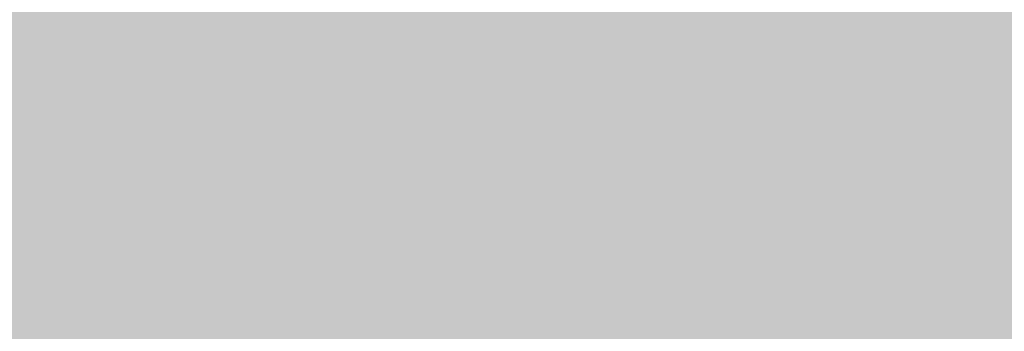
# Model space of a CAD drawing. Units: inches. Extents: x 2083 to 3317, y 1141 to 2115.
# Tile 142 of 256: x 3126.6699 to 3126.8176, y 1263.3081 to 1263.3548. Entities that reach past the tile are written whole.
import ezdxf

# ---------------------------------------------------------------- set-up
doc = ezdxf.new("R2010")
doc.units = ezdxf.units.IN
doc.layers.add('A-ANNO-DIMS', color=2, linetype='Continuous', lineweight=18)
doc.layers.add('A-WALL-PATT', color=251, linetype='Continuous', lineweight=13, true_color=0x636466)
doc.styles.get("Standard").update_dxf_attribs({"font": 'arial.ttf'})
doc.dimstyles.new('ISO-25', dxfattribs={"dimtxt": 12, "dimasz": 12, "dimexe": 1.25, "dimexo": 0.625, "dimtad": 1, "dimlunit": 3, "dimtxsty": 'Standard', "dimcen": 2.5, "dimadec": 0, "dimazin": 0, "dimtfac": 1, "dimtmove": 0, "dimatfit": 3, "dimfxl": 1, "dimarcsym": 0})

# ---------------------------------------------------------------- blocks, each defined once
blk = doc.blocks.new('*D26')
at = {"layer": 'A-ANNO-DIMS', "color": 0, "lineweight": -2, "transparency": 16777216}
for p, q in [((3088.98584, 1274.91509), (3088.98584, 1270.95196)), ((3111.24004, 1274.91509), (3111.24004, 1270.95196)), ((3076.98584, 1272.20196), (2840.26245, 1272.20196)), ((3111.24004, 1272.20196), (3088.98584, 1272.20196)), ((3123.24004, 1272.20196), (3135.24004, 1272.20196))]:
    blk.add_line(p, q, dxfattribs=at)
at = {"layer": 'A-ANNO-DIMS', "color": 0, "transparency": 16777216}
for points in [[(3076.98584, 1274.20196), (3076.98584, 1270.20196), (3088.98584, 1272.20196)], [(3123.24004, 1274.20196), (3123.24004, 1270.20196), (3111.24004, 1272.20196)]]:
    blk.add_solid(points, dxfattribs=at)
at = {"layer": 'Defpoints', "color": 0, "transparency": 16777216}
for p in [(3088.98584, 1275.54009), (3111.24004, 1275.54009), (3088.98584, 1272.20196)]:
    blk.add_point(p, dxfattribs=at)
at = {"layer": 'A-ANNO-DIMS', "color": 0, "transparency": 16777216, "insert": (2952.62415, 1279.0316), "char_height": 12, "attachment_point": 5}
blk.add_mtext('NIGHTSTAND 1\'-10 1/2" TYP.', dxfattribs=at)
blk = doc.blocks.new('*D27')
at = {"layer": 'A-ANNO-DIMS', "color": 0, "lineweight": -2, "transparency": 16777216}
for p, q in [((3114.57817, 1309.79428), (3114.57817, 1321.79428)), ((3111.86504, 1297.79428), (3115.82817, 1297.79428)), ((3114.57817, 1297.79428), (3114.57817, 1275.54009)), ((3111.86504, 1275.54009), (3115.82817, 1275.54009)), ((3114.57817, 1263.54009), (3114.57817, 1140.98859))]:
    blk.add_line(p, q, dxfattribs=at)
at = {"layer": 'A-ANNO-DIMS', "color": 0, "transparency": 16777216}
for points in [[(3112.57817, 1309.79428), (3116.57817, 1309.79428), (3114.57817, 1297.79428)], [(3112.57817, 1263.54009), (3116.57817, 1263.54009), (3114.57817, 1275.54009)]]:
    blk.add_solid(points, dxfattribs=at)
at = {"layer": 'Defpoints', "color": 0, "transparency": 16777216}
for p in [(3111.24004, 1297.79428), (3111.24004, 1275.54009), (3114.57817, 1275.54009)]:
    blk.add_point(p, dxfattribs=at)
at = {"layer": 'A-ANNO-DIMS', "color": 0, "transparency": 16777216, "insert": (3107.74853, 1196.26434), "char_height": 12, "attachment_point": 5, "rotation": 90}
blk.add_mtext('1\'-10 1/2" TYP.', dxfattribs=at)

msp = doc.modelspace()

# ---------------------------------------------------------------- hatches: boundary and pattern name
at = {"layer": 'A-WALL-PATT'}
h = msp.add_hatch(color=256, dxfattribs=at)
h.dxf.hatch_style = 1
h.paths.add_polyline_path([(3126.95978, 2020.76136), (2748.95978, 2020.76136), (2604.95978, 2020.76136), (2226.95978, 2020.76136), (2226.95978, 1702.76136), (2466.95978, 1702.76136), (2466.95978, 1582.76136), (2418.95978, 1582.76136), (2418.95978, 1477.76136), (2226.95978, 1477.76136), (2226.95978, 1263.26136), (2544.95978, 1263.26136), (2544.95978, 1411.76136), (2604.95978, 1411.76136), (2685.95978, 1411.76136), (2685.95978, 1420.76136), (2604.95978, 1420.76136), (2604.95978, 1573.76136), (2604.95978, 1702.76136), (2604.95978, 2011.76136), (2748.95978, 2011.76136), (2748.95978, 1702.76136), (2862.95978, 1702.76136), (2862.95978, 1621.76136), (2871.95978, 1621.76136), (2871.95978, 1702.76136), (2883.95978, 1702.76136), (2883.95978, 1706.93946, -0.026459), (2883.95978, 1711.76136), (2757.95978, 1711.76136), (2757.95978, 1807.76136), (2787.95978, 1807.76136), (2787.95978, 1812.26136), (2757.95978, 1812.26136), (2757.95978, 2011.76136), (2877.95978, 2011.76136), (2877.95978, 1812.26136), (2847.95978, 1812.26136), (2847.95978, 1807.76136), (2889.83574, 1807.76136), (2889.83574, 1812.26136), (2882.45978, 1812.26136), (2882.45978, 2011.76136), (3117.95978, 2011.76136), (3117.95978, 1812.26136), (2937.83574, 1812.26136), (2937.83574, 1807.76136), (2995.70978, 1807.76136), (2995.70978, 1796.11767), (3000.20978, 1796.11767), (3000.20978, 1807.76136), (3117.95978, 1807.76136), (3117.95978, 1711.76136), (3000.20978, 1711.76136), (3000.20978, 1760.11767), (2998.5727, 1760.11767, -0.020711), (2995.70978, 1760.11767), (2995.70978, 1711.76136), (2931.95978, 1711.76136), (2931.95978, 1702.76136), (3126.95978, 1702.76136)])
h.paths.add_polyline_path([(2471.45978, 2011.76136), (2471.45978, 1810.01136), (2462.71694, 1810.01136), (2462.71694, 1805.51136), (2505.95978, 1805.51136), (2505.95978, 1810.01136), (2475.95978, 1810.01136), (2475.95978, 2011.76136), (2595.95978, 2011.76136), (2595.95978, 1810.01136), (2565.95978, 1810.01136), (2565.95978, 1805.51136), (2595.95978, 1805.51136), (2595.95978, 1711.76136), (2235.95978, 1711.76136), (2235.95978, 1805.51136), (2353.70978, 1805.51136), (2353.70978, 1796.05416), (2358.20978, 1796.05416), (2358.20978, 1805.51136), (2414.71694, 1805.51136), (2414.71694, 1810.01136), (2235.95978, 1810.01136), (2235.95978, 2011.76136)], flags=16)
h.paths.add_polyline_path([(2270.20473, 1994.61001), (2270.20473, 1970.61001), (2246.20473, 1970.61001), (2246.20473, 1994.61001)], flags=0)
edge = h.paths.add_edge_path(flags=0)
edge.add_ellipse((2332.02739, 1899.79818), major_axis=(-3.04299, 3.04299), ratio=0.1682525, start_angle=-161.33217, end_angle=-156.30711, ccw=False)
edge.add_ellipse((2333.08204, 1898.74353), major_axis=(-1.05465, 1.05465), ratio=0.4535321, start_angle=-123.37102, end_angle=-94.15911)
edge = h.paths.add_edge_path(flags=0)
edge.add_ellipse((2332.02739, 1968.87629), major_axis=(3.04299, 3.04299), ratio=0.1682525, start_angle=18.66783, end_angle=23.69289)
edge.add_spline(control_points=[(2332.9256, 1970.6911), (2332.22677, 1970.3361), (2330.89371, 1969.65891), (2328.41308, 1970.93214), (2327.20393, 1967.74871), (2324.7096, 1969.95559), (2322.53282, 1967.01235), (2320.01285, 1971.29581), (2317.68031, 1968.15784), (2316.04053, 1967.10205), (2315.4269, 1966.8096)], knot_values=[0, 0, 0, 0, 2.267059, 4.324559, 6.685584, 8.878641, 11.121502, 14.300359, 17.755284, 19.732645, 19.732645, 19.732645, 19.732645], degree=3, periodic=0)
edge.add_ellipse((2332.02739, 1968.87629), major_axis=(3.04299, 3.04299), ratio=0.1682525, start_angle=18.66783, end_angle=23.69289, ccw=False)
edge.add_ellipse((2333.08204, 1969.93094), major_axis=(1.05465, 1.05465), ratio=0.4535321, start_angle=56.62898, end_angle=85.84089, ccw=False)
edge = h.paths.add_edge_path(flags=0)
edge.add_spline(control_points=[(2296.42829, 1967.98791), (2293.6278, 1965.33631), (2287.70362, 1959.72709), (2299.74386, 1949.9957), (2294.53259, 1935.66853), (2290.57323, 1920.60351), (2293.39412, 1909.97369), (2296.18541, 1904.96654)], knot_values=[0.099185, 0.099185, 0.099185, 0.099185, 0.345301, 0.619822, 0.982653, 1.386093, 1.810555, 1.810555, 1.810555, 1.810555], degree=3, periodic=0)
edge.add_spline(control_points=[(2296.18541, 1904.96654), (2297.38358, 1902.6193), (2298.00097, 1901.94931), (2298.55297, 1901.46815)], knot_values=[0.006246, 0.006246, 0.006246, 0.006246, 0.055476, 0.055476, 0.055476, 0.055476], degree=3, periodic=0)
edge.add_spline(control_points=[(2298.55297, 1901.46815), (2297.25861, 1900.92322), (2295.22529, 1900.23213), (2293.06023, 1900.61421), (2292.10142, 1900.78841), (2292.08958, 1900.79057)], knot_values=[0.312835, 0.312835, 0.312835, 0.312835, 0.40178, 0.474987, 0.475903, 0.475903, 0.475903, 0.475903], degree=3, periodic=0)
edge.add_arc((2292.79365, 1904.66411), 3.93701, 215.4209, 259.69818, ccw=False)
edge.add_spline(control_points=[(2289.58531, 1902.3823), (2289.47665, 1902.53509), (2289.36848, 1902.68804), (2289.26086, 1902.84117)], knot_values=[0.102872, 0.102872, 0.102872, 0.102872, 0.116896, 0.116896, 0.116896, 0.116896], degree=3, periodic=0)
edge.add_spline(control_points=[(2289.26086, 1902.84117), (2288.6866, 1902.55019), (2287.64005, 1902.0199), (2285.88134, 1901.87395), (2283.85297, 1901.50435), (2281.71999, 1899.71054), (2278.46699, 1899.49294), (2276.15714, 1901.8832), (2272.25895, 1899.80407), (2267.77761, 1901.84318), (2262.24388, 1900.18403), (2257.41493, 1901.78206), (2254.31837, 1900.72612), (2253.17828, 1900.33734)], knot_values=[0, 0, 0, 0, 1.907977, 3.477176, 5.261074, 7.972851, 11.680248, 13.717921, 16.939592, 22.789562, 27.502503, 33.595215, 37.145618, 37.145618, 37.145618, 37.145618], degree=3, periodic=0)
edge.add_line((2253.17828, 1900.33734), (2250.24424, 1902.84117))
edge.add_line((2250.24424, 1902.84117), (2250.24424, 1965.8333))
edge.add_line((2250.24424, 1965.8333), (2253.17828, 1968.33712))
edge.add_spline(control_points=[(2253.17828, 1968.33712), (2254.31837, 1967.94835), (2257.41493, 1966.89241), (2262.24388, 1968.49043), (2267.77761, 1966.83128), (2271.52673, 1968.53722), (2273.87591, 1967.82829), (2274.2067, 1967.72764)], knot_values=[0, 0, 0, 0, 0.09018, 0.244935, 0.364644, 0.513233, 0.537855, 0.537855, 0.537855, 0.537855], degree=3, periodic=0)
edge.add_arc((2274.35289, 1963.79335), 3.93701, 72.05113, 92.12795, ccw=False)
edge.add_arc((2281.29693, 1985.23), 18.5963, 252.051134, 288.565722)
edge.add_arc((2292.31672, 1956.02888), 12.64608, 71.026788, 113.778218, ccw=False)
edge = h.paths.add_edge_path(flags=0)
edge.add_spline(control_points=[(2274.89941, 1951.85619), (2275.06616, 1951.61659), (2275.23269, 1951.37659), (2275.39799, 1951.13585)], knot_values=[1.409916, 1.409916, 1.409916, 1.409916, 1.43159, 1.43159, 1.43159, 1.43159], degree=3, periodic=0)
edge.add_spline(control_points=[(2275.39799, 1951.13585), (2275.79211, 1950.56189), (2276.17923, 1949.98377), (2276.54555, 1949.3971)], knot_values=[1.358238, 1.358238, 1.358238, 1.358238, 1.409916, 1.409916, 1.409916, 1.409916], degree=3, periodic=0)
edge.add_line((2276.54555, 1949.3971), (2277.43729, 1947.86218))
edge.add_spline(control_points=[(2277.43729, 1947.86218), (2276.30383, 1945.67311), (2274.6397, 1942.42688), (2274.63161, 1938.0939), (2272.79912, 1930.85155), (2274.35643, 1943.89705), (2275.94768, 1947.92336), (2276.54555, 1949.3971)], knot_values=[0.005632, 0.005632, 0.005632, 0.005632, 0.186014, 0.266002, 0.357087, 0.59639, 0.739732, 0.739732, 0.739732, 0.739732], degree=3, periodic=0)
edge.add_spline(control_points=[(2276.54555, 1949.3971), (2276.17923, 1949.98377), (2275.79211, 1950.56189), (2275.39799, 1951.13585)], knot_values=[1.358238, 1.358238, 1.358238, 1.358238, 1.409916, 1.409916, 1.409916, 1.409916], degree=3, periodic=0)
edge.add_spline(control_points=[(2275.39799, 1951.13585), (2274.9425, 1950.08045), (2274.20776, 1948.02527), (2273.9346, 1944.85148), (2272.46853, 1937.62749), (2273.46622, 1945.69647), (2274.70062, 1951.05947), (2274.89941, 1951.85619)], knot_values=[0.104364, 0.104364, 0.104364, 0.104364, 0.189636, 0.269624, 0.36071, 0.600013, 0.644622, 0.644622, 0.644622, 0.644622], degree=3, periodic=0)
h.paths.add_polyline_path([(2269.16751, 1963.12757, -0.357527), (2268.17063, 1960.97637, -0.092561), (2268.17063, 1939.43632, -0.357527), (2269.16751, 1937.28512, -0.357527), (2267.01631, 1938.282, -0.164785), (2254.68558, 1938.282, -0.357527), (2252.53438, 1937.28512, -0.357527), (2253.53126, 1939.43632, -0.092561), (2253.53126, 1960.97637, -0.357527), (2252.53438, 1963.12757, -0.357527), (2254.68558, 1962.13069, -0.164785), (2267.01631, 1962.13069, -0.357527)], flags=0)
h.paths.add_polyline_path([(2248.87407, 1967.8018), (2248.87407, 1957.02771), (2249.45778, 1957.02771), (2249.45778, 1911.64676), (2248.87407, 1911.64676), (2248.87407, 1900.87267), (2246.51186, 1900.87267, 0.197327), (2244.14966, 1902.45687), (2244.14966, 1966.21759, 0.197327), (2246.51186, 1967.8018)], flags=0)
h.paths.add_polyline_path([(2269.16751, 1931.38934, -0.357527), (2268.17063, 1929.23814, -0.092561), (2268.17063, 1907.6981, -0.357527), (2269.16751, 1905.54689, -0.357527), (2267.01631, 1906.54377, -0.164785), (2254.68558, 1906.54377, -0.357527), (2252.53438, 1905.54689, -0.357527), (2253.53126, 1907.6981, -0.092561), (2253.53126, 1929.23814, -0.357527), (2252.53438, 1931.38934, -0.357527), (2254.68558, 1930.39246, -0.164785), (2267.01631, 1930.39246, -0.357527)], flags=0)
edge = h.paths.add_edge_path(flags=0)
edge.add_spline(control_points=[(2276.19686, 1906.7237), (2276.16814, 1909.02893), (2276.11405, 1913.37185), (2270.59842, 1924.92498), (2273.90517, 1919.01278), (2275.92171, 1916.26206), (2275.47457, 1912.40215), (2277.25787, 1910.38062), (2276.69604, 1908.22504), (2276.64622, 1906.81302), (2276.61782, 1906.00841)], knot_values=[0, 0, 0, 0, 8.61026, 16.221274, 18.843057, 23.804898, 27.440828, 29.356102, 31.203478, 33.650687, 33.650687, 33.650687, 33.650687], degree=3, periodic=0)
edge.add_spline(control_points=[(2276.61782, 1906.00841), (2276.62331, 1905.62414), (2276.49774, 1904.62866), (2275.44178, 1903.85473), (2274.93731, 1903.08045), (2274.85908, 1902.84117)], knot_values=[0.156488, 0.156488, 0.156488, 0.156488, 0.184398, 0.231376, 0.250598, 0.250598, 0.250598, 0.250598], degree=3, periodic=0)
edge.add_line((2274.85908, 1902.84117), (2276.50598, 1902.84117))
edge.add_spline(control_points=[(2276.50598, 1902.84117), (2276.78831, 1903.08494), (2277.66507, 1904.1252), (2278.24954, 1904.34074), (2277.65387, 1908.52739), (2278.15567, 1906.22781), (2278.10046, 1905.28595), (2278.84667, 1904.06901), (2277.85679, 1903.41495), (2277.87419, 1902.99105), (2277.90356, 1902.84117)], knot_values=[0.059574, 0.059574, 0.059574, 0.059574, 0.080753, 0.103741, 0.16972, 0.176036, 0.207137, 0.240474, 0.262341, 0.27366, 0.27366, 0.27366, 0.27366], degree=3, periodic=0)
edge.add_line((2277.90356, 1902.84117), (2280.02983, 1902.84117))
edge.add_spline(control_points=[(2280.02983, 1902.84117), (2279.88822, 1903.0884), (2279.49926, 1903.98155), (2280.15228, 1905.93935), (2278.10362, 1909.65776), (2279.76239, 1907.18529), (2280.3279, 1904.87486), (2280.48511, 1903.48959), (2281.46327, 1903.24943), (2281.75834, 1902.9365), (2281.83404, 1902.84117)], knot_values=[0.013856, 0.013856, 0.013856, 0.013856, 0.034874, 0.088867, 0.107879, 0.126738, 0.158714, 0.193757, 0.217487, 0.226722, 0.226722, 0.226722, 0.226722], degree=3, periodic=0)
edge.add_spline(control_points=[(2281.83404, 1902.84117), (2281.78753, 1902.8267), (2281.64702, 1902.78299), (2281.39553, 1902.85949), (2281.08808, 1902.98524), (2280.72068, 1903.0609), (2280.33345, 1903.02573), (2280.12477, 1902.89888), (2280.02983, 1902.84117)], knot_values=[0, 0, 0, 0, 0.14413, 0.435517, 0.749276, 1.153046, 1.548371, 1.878348, 1.878348, 1.878348, 1.878348], degree=3, periodic=0)
edge.add_line((2280.02983, 1902.84117), (2277.90356, 1902.84117))
edge.add_spline(control_points=[(2277.90356, 1902.84117), (2277.89286, 1902.79586), (2277.8654, 1902.67964), (2277.60748, 1902.68748), (2277.27405, 1902.8007), (2276.83792, 1902.61977), (2276.58381, 1902.78926), (2276.50598, 1902.84117)], knot_values=[0, 0, 0, 0, 0.127189, 0.326199, 0.628009, 1.24357, 1.515331, 1.515331, 1.515331, 1.515331], degree=3, periodic=0)
edge.add_line((2276.50598, 1902.84117), (2274.85908, 1902.84117))
edge.add_spline(control_points=[(2274.85908, 1902.84117), (2274.81444, 1902.89859), (2274.72513, 1903.01345), (2274.49348, 1903.11897), (2274.24429, 1902.96054), (2273.93712, 1903.18494), (2273.61404, 1902.98314), (2273.40832, 1902.88304), (2273.32225, 1902.84117)], knot_values=[0, 0, 0, 0, 0.21843, 0.436957, 0.687977, 0.990379, 1.398396, 1.69185, 1.69185, 1.69185, 1.69185], degree=3, periodic=0)
edge.add_spline(control_points=[(2273.32225, 1902.84117), (2273.61674, 1903.44569), (2274.274, 1904.53825), (2276.02724, 1904.5737), (2276.20696, 1906.58364), (2276.19686, 1906.7237)], knot_values=[0.012227, 0.012227, 0.012227, 0.012227, 0.059472, 0.106218, 0.134458, 0.134458, 0.134458, 0.134458], degree=3, periodic=0)
h.paths.add_polyline_path([(2270.77605, 1897.78983), (2270.77605, 1873.78983), (2246.77605, 1873.78983), (2246.77605, 1897.78983)], flags=0)
h.paths.add_polyline_path([(2353.70978, 1760.00506), (2353.70978, 1760.05416), (2358.20978, 1760.05416, -0.033729)], flags=0)
h.paths.add_polyline_path([(2321.81912, 1737.52919), (2341.99533, 1737.52919, -0.414214), (2343.20327, 1736.32124), (2343.20327, 1721.0206, -0.414214), (2341.99533, 1719.81265), (2321.81912, 1719.81265, -0.414214), (2320.61117, 1721.0206), (2320.61117, 1736.32124, -0.414214)], flags=0)
h.paths.add_polyline_path([(2324.23501, 1736.32124), (2339.57944, 1736.32124, -0.414214), (2341.99533, 1733.90535), (2341.99533, 1725.44973, -0.414214), (2339.57944, 1723.03384), (2333.68059, 1723.03384), (2333.84532, 1722.04547, -0.870646), (2335.4254, 1721.82589, -0.767327), (2333.92269, 1721.42324), (2331.29102, 1721.42324, -0.767327), (2329.78832, 1721.82589, -0.870646), (2331.3684, 1722.04547), (2331.53313, 1723.03384), (2324.23501, 1723.03384, -0.414214), (2321.81912, 1725.44973), (2321.81912, 1733.90535, -0.414214)], flags=0)
h.paths.add_polyline_path([(2570.48379, 1928.61544), (2589.68379, 1928.61544), (2590.16883, 1928.61544), (2590.16883, 1904.9934), (2570.48379, 1904.9934)], flags=0)
h.paths.add_polyline_path([(2574.44732, 1927.26382, -1), (2572.82884, 1927.26382, -1)], flags=0)
h.paths.add_polyline_path([(2573.08987, 1926.94088), (2573.92503, 1927.77604), (2574.14774, 1927.55333), (2573.31258, 1926.71817)], flags=0)
h.paths.add_polyline_path([(2578.77906, 1919.72962, -1), (2571.59166, 1919.72962, -1)], flags=0)
h.paths.add_polyline_path([(2578.38536, 1919.72962, -1), (2571.98536, 1919.72962, -1)], flags=0)
h.paths.add_polyline_path([(2331.59576, 1729.47622, -1), (2333.61795, 1729.47622, -1)], flags=0)
h.paths.add_polyline_path([(2578.03423, 1927.26382, -1), (2576.41574, 1927.26382, -1)], flags=0)
h.paths.add_polyline_path([(2576.68885, 1927.53109), (2576.91156, 1927.7538), (2577.74673, 1926.91863), (2577.52402, 1926.69592)], flags=0)
h.paths.add_polyline_path([(2578.13906, 1909.85954, -1), (2572.23166, 1909.85954, -1)], flags=0)
h.paths.add_polyline_path([(2577.74536, 1909.85954, -1), (2572.62536, 1909.85954, -1)], flags=0)
h.paths.add_polyline_path([(2583.79772, 1927.26382, -1), (2582.17923, 1927.26382, -1)], flags=0)
h.paths.add_polyline_path([(2582.71865, 1927.7538), (2583.55381, 1926.91863), (2583.3311, 1926.69592), (2582.49594, 1927.53109)], flags=0)
h.paths.add_polyline_path([(2582.49594, 1927.53109), (2582.71865, 1927.7538), (2583.55381, 1926.91863), (2583.3311, 1926.69592)], flags=0)
h.paths.add_polyline_path([(2587.73906, 1920.52962, -1), (2581.83166, 1920.52962, -1)], flags=0)
h.paths.add_polyline_path([(2587.34536, 1920.52962, -1), (2582.22536, 1920.52962, -1)], flags=0)
h.paths.add_polyline_path([(2587.38462, 1927.26382, -1), (2585.76613, 1927.26382, -1)], flags=0)
h.paths.add_polyline_path([(2586.08199, 1926.98025), (2586.91716, 1927.81541), (2587.13987, 1927.5927), (2586.3047, 1926.75754)], flags=0)
h.paths.add_polyline_path([(2588.37906, 1910.65954, -1), (2581.19166, 1910.65954, -1)], flags=0)
h.paths.add_polyline_path([(2587.98536, 1910.65954, -1), (2581.58536, 1910.65954, -1)], flags=0)
h.paths.add_polyline_path([(2417.16773, 1729.4779), (2437.34394, 1729.4779, -0.414214), (2438.55188, 1728.26995), (2438.55188, 1712.96931, -0.414214), (2437.34394, 1711.76136), (2417.16773, 1711.76136, -0.414214), (2415.95978, 1712.96931), (2415.95978, 1728.26995, -0.414214)], flags=0)
h.paths.add_polyline_path([(2419.58362, 1728.26995), (2434.92805, 1728.26995, -0.414214), (2437.34394, 1725.85406), (2437.34394, 1717.39844, -0.414214), (2434.92805, 1714.98255), (2429.0292, 1714.98255), (2429.19393, 1713.99418, -0.870646), (2430.77401, 1713.7746, -0.767327), (2429.2713, 1713.37195), (2426.63963, 1713.37195, -0.767327), (2425.13693, 1713.7746, -0.870646), (2426.71701, 1713.99418), (2426.88174, 1714.98255), (2419.58362, 1714.98255, -0.414214), (2417.16773, 1717.39844), (2417.16773, 1725.85406, -0.414214)], flags=0)
h.paths.add_polyline_path([(2419.58362, 1728.26995), (2434.92805, 1728.26995, -0.414214), (2437.34394, 1725.85406), (2437.34394, 1717.39844, -0.414214), (2434.92805, 1714.98255), (2429.0292, 1714.98255), (2428.35812, 1719.00903), (2427.55282, 1719.00903), (2426.88174, 1714.98255), (2419.58362, 1714.98255, -0.414214), (2417.16773, 1717.39844), (2417.16773, 1725.85406, -0.414214)], flags=0)
h.paths.add_polyline_path([(2426.94437, 1721.42492, -1), (2428.96656, 1721.42492, -1)], flags=0)
h.paths.add_polyline_path([(2475.95978, 1702.76136), (2595.95978, 1702.76136), (2595.95978, 1582.76136), (2475.95978, 1582.76136)], flags=16)
h.paths.add_polyline_path([(2427.95978, 1573.76136), (2595.95978, 1573.76136), (2595.95978, 1468.76136), (2595.95978, 1420.76136), (2384.45978, 1420.76136), (2384.45978, 1468.76136), (2427.95978, 1468.76136)], flags=16)
h.paths.add_polyline_path([(2379.95978, 1468.76136), (2379.95978, 1420.76136), (2235.95978, 1420.76136), (2235.95978, 1468.76136)], flags=16)
h.paths.add_polyline_path([(2317.816, 1466.69577), (2337.9922, 1466.69577, -0.414214), (2339.20015, 1465.48782), (2339.20015, 1450.18718, -0.414214), (2337.9922, 1448.97923), (2317.816, 1448.97923, -0.414214), (2316.60805, 1450.18718), (2316.60805, 1465.48782, -0.414214)], flags=0)
h.paths.add_polyline_path([(2320.23189, 1465.48782), (2335.57631, 1465.48782, -0.414214), (2337.9922, 1463.07193), (2337.9922, 1454.61631, -0.414214), (2335.57631, 1452.20042), (2329.67747, 1452.20042), (2329.84219, 1451.21205, -0.870646), (2331.42228, 1450.99247, -0.767327), (2329.91957, 1450.58983), (2327.2879, 1450.58983, -0.767327), (2325.7852, 1450.99247, -0.870646), (2327.36528, 1451.21205), (2327.53001, 1452.20042), (2320.23189, 1452.20042, -0.414214), (2317.816, 1454.61631), (2317.816, 1463.07193, -0.414214)], flags=0)
h.paths.add_polyline_path([(2320.23189, 1465.48782), (2335.57631, 1465.48782, -0.414214), (2337.9922, 1463.07193), (2337.9922, 1454.61631, -0.414214), (2335.57631, 1452.20042), (2329.67747, 1452.20042), (2329.00638, 1456.22691), (2328.20109, 1456.22691), (2327.53001, 1452.20042), (2320.23189, 1452.20042, -0.414214), (2317.816, 1454.61631), (2317.816, 1463.07193, -0.414214)], flags=0)
h.paths.add_polyline_path([(2327.59264, 1458.6428, -1), (2329.61483, 1458.6428, -1)], flags=0)
h.paths.add_polyline_path([(2244.41174, 1433.34045), (2241.92094, 1433.34045, -0.414214), (2240.01786, 1435.24354), (2240.01786, 1440.95281, -0.414211), (2241.92093, 1442.8559), (2244.41174, 1442.8559, -1.976472)], flags=0)
h.paths.add_polyline_path([(2245.35689, 1434.39754, -0.414214), (2245.35689, 1441.79881, -2.144098)], flags=0)
h.paths.add_polyline_path([(2535.95978, 1416.26136), (2535.95978, 1272.26136), (2235.95978, 1272.26136), (2235.95978, 1416.26136)], flags=16)
h.paths.add_polyline_path([(2260.11956, 1384.29284), (2260.11956, 1362.03865), (2237.86537, 1362.03865), (2237.86537, 1384.29284)], flags=0)
edge = h.paths.add_edge_path(flags=0)
edge.add_line((2318.25185, 1362.0933), (2318.1458, 1362.00097))
edge.add_ellipse((2317.44512, 1360.43104), major_axis=(2.82164, 2.82164), ratio=0.1682525, start_angle=18.66783, end_angle=20.94813, ccw=False)
edge.add_ellipse((2318.42305, 1361.40897), major_axis=(0.97793, 0.97793), ratio=0.4535321, start_angle=56.62898, end_angle=70.2262, ccw=False)
edge = h.paths.add_edge_path(flags=0)
edge.add_line((2319.10737, 1295.57108), (2319.01504, 1295.67713))
edge.add_ellipse((2317.44512, 1296.37781), major_axis=(-2.82164, 2.82164), ratio=0.1682525, start_angle=-161.33217, end_angle=-159.05187, ccw=False)
edge.add_ellipse((2318.42305, 1295.39988), major_axis=(-0.97793, 0.97793), ratio=0.4535321, start_angle=-123.37102, end_angle=-109.7738)
edge = h.paths.add_edge_path(flags=0)
edge.add_spline(control_points=[(2284.21035, 1301.17022), (2284.58069, 1300.44472), (2284.89119, 1299.89202), (2285.15955, 1299.46102)], knot_values=[0.039066, 0.039066, 0.039066, 0.039066, 0.055476, 0.055476, 0.055476, 0.055476], degree=3, periodic=0)
edge.add_line((2285.15955, 1299.46102), (2284.21035, 1301.17022))
edge = h.paths.add_edge_path(flags=0)
edge.add_line((2280.41246, 1297.29801), (2283.36999, 1297.03612))
edge.add_line((2283.36999, 1297.03612), (2286.40569, 1297.92631))
edge.add_spline(control_points=[(2286.40569, 1297.92631), (2285.30549, 1297.46312), (2284.34478, 1297.12915), (2283.36999, 1297.03612)], knot_values=[0.394369, 0.394369, 0.394369, 0.394369, 0.475903, 0.475903, 0.475903, 0.475903], degree=3, periodic=0)
edge.add_spline(control_points=[(2283.36999, 1297.03612), (2283.28139, 1297.02767), (2282.31629, 1296.95734), (2281.3125, 1297.13448), (2280.42344, 1297.29602), (2280.41246, 1297.29801)], knot_values=[0.312835, 0.312835, 0.312835, 0.312835, 0.320246, 0.393453, 0.394369, 0.394369, 0.394369, 0.394369], degree=3, periodic=0)
edge = h.paths.add_edge_path(flags=0)
edge.add_line((2284.43556, 1359.60729), (2280.44629, 1355.32805))
edge.add_line((2280.44629, 1355.32805), (2279.57999, 1351.01775))
edge.add_line((2279.57999, 1351.01775), (2282.41297, 1346.58043))
edge.add_spline(control_points=[(2282.41297, 1346.58043), (2283.15333, 1345.58924), (2284.2529, 1344.0289), (2284.80104, 1342.38717), (2284.93516, 1341.80554)], knot_values=[1.240098, 1.240098, 1.240098, 1.240098, 1.332892, 1.382712, 1.382712, 1.382712, 1.382712], degree=3, periodic=0)
edge.add_spline(control_points=[(2284.93516, 1341.80554), (2285.31911, 1340.1406), (2285.23303, 1338.4092), (2284.90994, 1336.65412)], knot_values=[1.097484, 1.097484, 1.097484, 1.097484, 1.240098, 1.240098, 1.240098, 1.240098], degree=3, periodic=0)
edge.add_spline(control_points=[(2284.90994, 1336.65412), (2284.58685, 1334.89904), (2284.02675, 1333.12027), (2283.46264, 1331.36058)], knot_values=[0.95487, 0.95487, 0.95487, 0.95487, 1.097484, 1.097484, 1.097484, 1.097484], degree=3, periodic=0)
edge.add_line((2283.46264, 1331.36058), (2281.89038, 1326.15336))
edge.add_line((2281.89038, 1326.15336), (2280.75626, 1321.05609))
edge.add_line((2280.75626, 1321.05609), (2280.2992, 1316.00198))
edge.add_line((2280.2992, 1316.00198), (2280.71593, 1310.95007))
edge.add_line((2280.71593, 1310.95007), (2282.02809, 1305.97214))
edge.add_line((2282.02809, 1305.97214), (2284.21035, 1301.17022))
edge.add_spline(control_points=[(2284.21035, 1301.17022), (2283.34073, 1302.73019), (2282.6119, 1304.33649), (2282.02809, 1305.97214)], knot_values=[0.099185, 0.099185, 0.099185, 0.099185, 0.241799, 0.241799, 0.241799, 0.241799], degree=3, periodic=0)
edge.add_spline(control_points=[(2282.02809, 1305.97214), (2281.44428, 1307.60778), (2281.00549, 1309.27276), (2280.71593, 1310.95007)], knot_values=[0.241799, 0.241799, 0.241799, 0.241799, 0.384413, 0.384413, 0.384413, 0.384413], degree=3, periodic=0)
edge.add_spline(control_points=[(2280.71593, 1310.95007), (2280.43324, 1312.58761), (2280.28939, 1314.27696), (2280.29889, 1315.96203), (2280.2992, 1316.00198)], knot_values=[0.384413, 0.384413, 0.384413, 0.384413, 0.523647, 0.527028, 0.527028, 0.527028, 0.527028], degree=3, periodic=0)
edge.add_spline(control_points=[(2280.2992, 1316.00198), (2280.31233, 1317.68696), (2280.47787, 1319.36793), (2280.75626, 1321.05609)], knot_values=[0.527028, 0.527028, 0.527028, 0.527028, 0.669642, 0.669642, 0.669642, 0.669642], degree=3, periodic=0)
edge.add_spline(control_points=[(2280.75626, 1321.05609), (2281.03465, 1322.74425), (2281.42588, 1324.43961), (2281.89038, 1326.15336)], knot_values=[0.669642, 0.669642, 0.669642, 0.669642, 0.812256, 0.812256, 0.812256, 0.812256], degree=3, periodic=0)
edge.add_spline(control_points=[(2281.89038, 1326.15336), (2282.26438, 1327.53325), (2282.78787, 1329.26181), (2283.35275, 1331.01778), (2283.46264, 1331.36058)], knot_values=[0.812256, 0.812256, 0.812256, 0.812256, 0.927087, 0.95487, 0.95487, 0.95487, 0.95487], degree=3, periodic=0)
edge.add_line((2283.46264, 1331.36058), (2284.90994, 1336.65412))
edge.add_line((2284.90994, 1336.65412), (2284.93516, 1341.80554))
edge.add_line((2284.93516, 1341.80554), (2282.41297, 1346.58043))
edge.add_spline(control_points=[(2282.41297, 1346.58043), (2281.27513, 1348.10379), (2280.07845, 1349.57032), (2279.57999, 1351.01775)], knot_values=[1.382712, 1.382712, 1.382712, 1.382712, 1.525326, 1.525326, 1.525326, 1.525326], degree=3, periodic=0)
edge.add_spline(control_points=[(2279.57999, 1351.01775), (2279.44328, 1351.41472), (2279.13631, 1352.85692), (2279.73519, 1354.29039), (2280.44629, 1355.32805)], knot_values=[1.525326, 1.525326, 1.525326, 1.525326, 1.564439, 1.667941, 1.667941, 1.667941, 1.667941], degree=3, periodic=0)
edge.add_spline(control_points=[(2280.44629, 1355.32805), (2281.42611, 1356.75784), (2282.93084, 1358.18256), (2284.43556, 1359.60729)], knot_values=[1.667941, 1.667941, 1.667941, 1.667941, 1.810555, 1.810555, 1.810555, 1.810555], degree=3, periodic=0)
edge.add_arc((2280.62307, 1348.51818), 11.72618, 71.026788, 113.778218)
edge.add_arc((2270.40489, 1375.59516), 17.24357, 252.051134, 288.565722, ccw=False)
edge.add_arc((2263.96597, 1355.71785), 3.65062, 72.05113, 92.12795)
edge.add_arc((2263.96597, 1355.71785), 3.65062, 92.12795, 177.98513)
edge.add_spline(control_points=[(2260.3176, 1355.8462), (2260.26042, 1354.22067), (2260.55128, 1350.18655), (2262.99934, 1346.76625), (2264.47274, 1344.64902)], knot_values=[1.43159, 1.43159, 1.43159, 1.43159, 1.564144, 1.770695, 1.770695, 1.770695, 1.770695], degree=3, periodic=0)
edge.add_line((2264.47274, 1344.64902), (2264.93559, 1343.98253))
edge.add_spline(control_points=[(2263.80104, 1340.24811), (2263.84324, 1340.51409), (2264.06724, 1341.75647), (2264.51269, 1343.00245), (2264.93505, 1343.98108)], knot_values=[0.53657, 0.53657, 0.53657, 0.53657, 0.559349, 0.644622, 0.644622, 0.644622, 0.644622], degree=3, periodic=0)
edge.add_spline(control_points=[(2264.93505, 1343.98108), (2265.11777, 1343.71497), (2265.29888, 1343.44791), (2265.47676, 1343.17936)], knot_values=[1.384077, 1.384077, 1.384077, 1.384077, 1.409916, 1.409916, 1.409916, 1.409916], degree=3, periodic=0)
edge.add_spline(control_points=[(2265.47676, 1343.17936), (2265.65464, 1342.91082), (2265.8293, 1342.64081), (2265.99913, 1342.36881)], knot_values=[1.358238, 1.358238, 1.358238, 1.358238, 1.384077, 1.384077, 1.384077, 1.384077], degree=3, periodic=0)
edge.add_line((2265.99913, 1342.36881), (2266.82601, 1340.94555))
edge.add_spline(control_points=[(2266.82601, 1340.94555), (2268.8944, 1337.08969), (2271.39817, 1325.843), (2270.51616, 1310.56856), (2275.91938, 1301.86061), (2277.78951, 1299.19945)], knot_values=[0.116896, 0.116896, 0.116896, 0.116896, 0.472987, 1.050969, 1.313793, 1.313793, 1.313793, 1.313793], degree=3, periodic=0)
edge.add_spline(control_points=[(2277.78951, 1299.19945), (2277.83941, 1299.12845), (2277.88943, 1299.0575), (2277.93957, 1298.98658)], knot_values=[0.109884, 0.109884, 0.109884, 0.109884, 0.116896, 0.116896, 0.116896, 0.116896], degree=3, periodic=0)
edge.add_line((2277.93957, 1298.98658), (2277.78885, 1299.19911))
edge.add_spline(control_points=[(2277.78885, 1299.19911), (2277.25658, 1298.92941), (2276.28635, 1298.4379), (2275.03935, 1298.33442), (2274.38333, 1298.2389), (2274.21525, 1298.20934)], knot_values=[33.12187, 33.12187, 33.12187, 33.12187, 35.029056, 36.598255, 37.144827, 37.144827, 37.144827, 37.144827], degree=3, periodic=0)
edge.add_line((2274.21525, 1298.20934), (2273.07315, 1297.89296))
edge.add_spline(control_points=[(2273.07315, 1297.89296), (2272.32294, 1297.57978), (2271.03915, 1296.51051), (2269.24839, 1296.22606), (2268.4231, 1296.37465)], knot_values=[26.532584, 26.532584, 26.532584, 26.532584, 29.198919, 31.839101, 31.839101, 31.839101, 31.839101], degree=3, periodic=0)
edge.add_line((2268.4231, 1296.37465), (2263.8785, 1297.45753))
edge.add_spline(control_points=[(2263.8785, 1297.45753), (2263.55608, 1297.35943), (2261.86031, 1296.83869), (2260.23878, 1297.28241), (2258.93345, 1297.51646)], knot_values=[15.919551, 15.919551, 15.919551, 15.919551, 16.939592, 21.226067, 21.226067, 21.226067, 21.226067], degree=3, periodic=0)
edge.add_line((2258.93345, 1297.51646), (2254.05523, 1297.32901))
edge.add_spline(control_points=[(2254.05523, 1297.32901), (2253.75553, 1297.29582), (2252.11368, 1297.16517), (2250.46187, 1297.54422), (2249.12969, 1297.66788)], knot_values=[5.306517, 5.306517, 5.306517, 5.306517, 6.276435, 10.613034, 10.613034, 10.613034, 10.613034], degree=3, periodic=0)
edge.add_line((2249.12969, 1297.66788), (2244.33165, 1296.87776))
edge.add_line((2244.33165, 1296.87776), (2241.61103, 1299.19945))
edge.add_line((2241.61103, 1299.19945), (2241.61103, 1357.6094))
edge.add_line((2241.61103, 1357.6094), (2244.33165, 1359.9311))
edge.add_line((2244.33165, 1359.9311), (2252.72882, 1359.54269))
edge.add_spline(control_points=[(2252.72882, 1359.54269), (2252.87094, 1359.54644), (2253.30574, 1359.54817), (2253.73984, 1359.51427), (2254.03174, 1359.48243)], knot_values=[0.233291, 0.233291, 0.233291, 0.233291, 0.244935, 0.268927, 0.268927, 0.268927, 0.268927], degree=3, periodic=0)
edge.add_line((2254.03174, 1359.48243), (2259.58719, 1359.41639))
edge.add_spline(control_points=[(2259.58719, 1359.41639), (2260.67707, 1359.6285), (2262.0732, 1359.897), (2263.52369, 1359.45928), (2263.83042, 1359.36595)], knot_values=[0.422516, 0.422516, 0.422516, 0.422516, 0.513233, 0.537855, 0.537855, 0.537855, 0.537855], degree=3, periodic=0)
edge.add_arc((2263.96597, 1355.71785), 3.65062, 72.05113, 92.12795, ccw=False)
edge.add_arc((2270.40489, 1375.59516), 17.24357, 252.051134, 288.565722)
edge.add_arc((2280.62307, 1348.51818), 11.72618, 71.026788, 113.778218, ccw=False)
h.paths.add_polyline_path([(2240.34053, 1359.43471), (2240.34053, 1349.44435), (2240.88178, 1349.44435), (2240.88178, 1307.3645), (2240.34053, 1307.3645), (2240.34053, 1297.37414), (2238.15016, 1297.37414, 0.197327), (2235.95978, 1298.84311), (2235.95978, 1357.96575, 0.197327), (2238.15016, 1359.43471)], flags=0)
h.paths.add_polyline_path([(2259.15779, 1355.1005, -0.357527), (2258.23342, 1353.10578, -0.092561), (2258.23342, 1333.1326, -0.357527), (2259.15779, 1331.13788, -0.357527), (2257.16307, 1332.06225, -0.164785), (2245.7293, 1332.06225, -0.357527), (2243.73458, 1331.13788, -0.357527), (2244.65895, 1333.1326, -0.092561), (2244.65895, 1353.10578, -0.357527), (2243.73458, 1355.1005, -0.357527), (2245.7293, 1354.17613, -0.164785), (2257.16307, 1354.17613, -0.357527)], flags=0)
edge = h.paths.add_edge_path(flags=0)
edge.add_line((2265.99913, 1342.36881), (2266.82601, 1340.94555))
edge.add_line((2266.82601, 1340.94555), (2265.30756, 1337.81407))
edge.add_line((2265.30756, 1337.81407), (2264.35823, 1334.65294))
edge.add_line((2264.35823, 1334.65294), (2264.26201, 1333.7997))
edge.add_spline(control_points=[(2264.26201, 1333.7997), (2264.20836, 1333.18705), (2264.16206, 1332.36553), (2264.00714, 1331.41393), (2263.96905, 1331.20183)], knot_values=[0.464444, 0.464444, 0.464444, 0.464444, 0.516691, 0.531608, 0.531608, 0.531608, 0.531608], degree=3, periodic=0)
edge.add_spline(control_points=[(2263.96905, 1331.20183), (2263.77453, 1330.11887), (2263.42437, 1328.79084), (2263.25742, 1328.53065), (2263.23403, 1328.51461)], knot_values=[0.372682, 0.372682, 0.372682, 0.372682, 0.44885, 0.464444, 0.464444, 0.464444, 0.464444], degree=3, periodic=0)
edge.add_spline(control_points=[(2263.23403, 1328.51461), (2263.09638, 1328.42023), (2263.13117, 1329.30148), (2263.27495, 1330.61575)], knot_values=[0.280919, 0.280919, 0.280919, 0.280919, 0.372682, 0.372682, 0.372682, 0.372682], degree=3, periodic=0)
edge.add_spline(control_points=[(2263.27495, 1330.61575), (2263.41874, 1331.93002), (2263.67152, 1333.67732), (2263.96985, 1335.31503)], knot_values=[0.189157, 0.189157, 0.189157, 0.189157, 0.280919, 0.280919, 0.280919, 0.280919], degree=3, periodic=0)
edge.add_spline(control_points=[(2263.96985, 1335.31503), (2264.1005, 1336.03219), (2264.41878, 1337.62191), (2264.75485, 1338.86443), (2264.94742, 1339.49112)], knot_values=[0.097394, 0.097394, 0.097394, 0.097394, 0.137578, 0.189157, 0.189157, 0.189157, 0.189157], degree=3, periodic=0)
edge.add_spline(control_points=[(2264.94742, 1339.49112), (2265.29002, 1340.60605), (2265.64424, 1341.494), (2265.99913, 1342.36881)], knot_values=[0.005632, 0.005632, 0.005632, 0.005632, 0.097394, 0.097394, 0.097394, 0.097394], degree=3, periodic=0)
h.paths.add_polyline_path([(2259.15779, 1325.67097, -0.357527), (2258.23342, 1323.67625, -0.092561), (2258.23342, 1303.70307, -0.357527), (2259.15779, 1301.70835, -0.357527), (2257.16307, 1302.63272, -0.164785), (2245.7293, 1302.63272, -0.357527), (2243.73458, 1301.70835, -0.357527), (2244.65895, 1303.70307, -0.092561), (2244.65895, 1323.67625, -0.357527), (2243.73458, 1325.67097, -0.357527), (2245.7293, 1324.74661, -0.164785), (2257.16307, 1324.74661, -0.357527)], flags=0)
edge = h.paths.add_edge_path(flags=0)
edge.add_spline(control_points=[(2261.70894, 1317.31142), (2261.67948, 1317.41758), (2261.76186, 1317.38853), (2262.49074, 1316.08987), (2262.96218, 1315.3009)], knot_values=[14.955861, 14.955861, 14.955861, 14.955861, 16.221274, 18.694826, 18.694826, 18.694826, 18.694826], degree=3, periodic=0)
edge.add_spline(control_points=[(2262.96218, 1315.3009), (2262.99044, 1315.25362), (2263.7021, 1314.06738), (2264.34898, 1313.12715), (2264.73005, 1312.16415)], knot_values=[18.694826, 18.694826, 18.694826, 18.694826, 18.843057, 22.433791, 22.433791, 22.433791, 22.433791], degree=3, periodic=0)
edge.add_spline(control_points=[(2264.73005, 1312.16415), (2264.87556, 1311.79644), (2265.17687, 1310.76981), (2265.14307, 1309.55926), (2265.24774, 1308.82419)], knot_values=[22.433791, 22.433791, 22.433791, 22.433791, 23.804898, 26.172756, 26.172756, 26.172756, 26.172756], degree=3, periodic=0)
edge.add_line((2265.24774, 1308.82419), (2265.85077, 1307.17189))
edge.add_spline(control_points=[(2265.85077, 1307.17189), (2266.06502, 1306.82168), (2266.38439, 1306.33225), (2266.4244, 1305.78055), (2266.42037, 1305.61122)], knot_values=[28.062562, 28.062562, 28.062562, 28.062562, 29.356102, 29.911721, 29.911721, 29.911721, 29.911721], degree=3, periodic=0)
edge.add_spline(control_points=[(2266.42037, 1305.61122), (2266.41612, 1305.43259), (2266.394, 1305.25), (2266.36478, 1305.06586)], knot_values=[29.911721, 29.911721, 29.911721, 29.911721, 30.497837, 30.497837, 30.497837, 30.497837], degree=3, periodic=0)
edge.add_line((2266.36478, 1305.06586), (2266.06615, 1302.1363))
edge.add_spline(control_points=[(2266.06615, 1302.1363), (2266.07124, 1301.77998), (2265.99808, 1301.19998), (2265.66327, 1300.75896), (2265.50891, 1300.58588)], knot_values=[0.156488, 0.156488, 0.156488, 0.156488, 0.184398, 0.203543, 0.203543, 0.203543, 0.203543], degree=3, periodic=0)
edge.add_line((2265.50891, 1300.58588), (2264.43534, 1299.19945))
edge.add_line((2264.43534, 1299.19945), (2265.96244, 1299.19945))
edge.add_line((2265.96244, 1299.19945), (2267.33599, 1301.17528))
edge.add_line((2267.33599, 1301.17528), (2267.31167, 1301.98624))
edge.add_spline(control_points=[(2267.31167, 1301.98624), (2267.26111, 1302.8624), (2267.16021, 1303.73713), (2267.27149, 1303.3259)], knot_values=[0.126229, 0.126229, 0.126229, 0.126229, 0.166617, 0.166617, 0.166617, 0.166617], degree=3, periodic=0)
edge.add_spline(control_points=[(2267.27149, 1303.3259), (2267.28003, 1303.2943), (2267.30979, 1303.17537), (2267.37345, 1302.88361), (2267.40612, 1302.68283), (2267.41793, 1302.60103)], knot_values=[0.166617, 0.166617, 0.166617, 0.166617, 0.16972, 0.176036, 0.180765, 0.180765, 0.180765, 0.180765], degree=3, periodic=0)
edge.add_spline(control_points=[(2267.74389, 1300.9875), (2267.68758, 1301.15094), (2267.48052, 1301.65666), (2267.48375, 1302.14479), (2267.41793, 1302.60103)], knot_values=[0.180765, 0.180765, 0.180765, 0.180765, 0.193767, 0.220139, 0.220139, 0.220139, 0.220139], degree=3, periodic=0)
edge.add_line((2267.41793, 1302.60103), (2267.74389, 1300.9875))
edge.add_spline(control_points=[(2267.74389, 1300.9875), (2267.83196, 1300.73188), (2267.93202, 1300.3099), (2267.55484, 1299.97452), (2267.42937, 1299.82921)], knot_values=[0.220139, 0.220139, 0.220139, 0.220139, 0.240474, 0.25489, 0.25489, 0.25489, 0.25489], degree=3, periodic=0)
edge.add_line((2267.42937, 1299.82921), (2267.25836, 1299.19945))
edge.add_line((2267.25836, 1299.19945), (2269.22996, 1299.19945))
edge.add_spline(control_points=[(2269.22996, 1299.19945), (2269.09865, 1299.42869), (2268.84277, 1300.01625), (2269.01157, 1300.91592), (2268.9468, 1301.66074)], knot_values=[0.013856, 0.013856, 0.013856, 0.013856, 0.034874, 0.067073, 0.067073, 0.067073, 0.067073], degree=3, periodic=0)
edge.add_line((2268.9468, 1301.66074), (2268.43158, 1303.60311))
edge.add_spline(control_points=[(2268.43158, 1303.60311), (2268.1756, 1304.19237), (2267.59621, 1305.2513), (2268.0407, 1304.62321), (2268.25139, 1304.28242)], knot_values=[0.090155, 0.090155, 0.090155, 0.090155, 0.107879, 0.120289, 0.120289, 0.120289, 0.120289], degree=3, periodic=0)
edge.add_spline(control_points=[(2268.25139, 1304.28242), (2268.36088, 1304.10533), (2269.05775, 1302.91798), (2269.38269, 1301.59042), (2269.52141, 1300.77593), (2269.57522, 1300.55578)], knot_values=[0.120289, 0.120289, 0.120289, 0.120289, 0.126738, 0.158714, 0.173506, 0.173506, 0.173506, 0.173506], degree=3, periodic=0)
edge.add_line((2269.57522, 1300.55578), (2270.6858, 1299.42126))
edge.add_spline(control_points=[(2270.6858, 1299.42126), (2270.76722, 1299.35725), (2270.83785, 1299.2814), (2270.90292, 1299.19945)], knot_values=[0.21816, 0.21816, 0.21816, 0.21816, 0.226722, 0.226722, 0.226722, 0.226722], degree=3, periodic=0)
edge.add_line((2270.9372, 1299.19291), (2270.90292, 1299.19945))
edge.add_spline(control_points=[(2270.90292, 1299.19945), (2270.85981, 1299.18603), (2270.72951, 1299.1455), (2270.49631, 1299.21644), (2270.27166, 1299.30832), (2270.12102, 1299.34796), (2270.06334, 1299.35956)], knot_values=[0.939174, 0.939174, 0.939174, 0.939174, 1.083304, 1.374691, 1.68845, 1.878348, 1.878348, 1.878348, 1.878348], degree=3, periodic=0)
edge.add_line((2270.06334, 1299.35956), (2269.22996, 1299.19945))
edge.add_line((2269.22996, 1299.19945), (2267.25836, 1299.19945))
edge.add_spline(control_points=[(2267.25836, 1299.19945), (2267.24843, 1299.15743), (2267.22297, 1299.04967), (2266.98382, 1299.05694), (2266.80921, 1299.11623), (2266.6769, 1299.10909), (2266.63653, 1299.10481)], knot_values=[0.757665, 0.757665, 0.757665, 0.757665, 0.884854, 1.083864, 1.385675, 1.515331, 1.515331, 1.515331, 1.515331], degree=3, periodic=0)
edge.add_spline(control_points=[(2266.63653, 1299.10481), (2266.48522, 1299.08879), (2266.23581, 1299.01712), (2266.03461, 1299.15132), (2265.96244, 1299.19945)], knot_values=[0, 0, 0, 0, 0.485905, 0.757665, 0.757665, 0.757665, 0.757665], degree=3, periodic=0)
edge.add_line((2265.96244, 1299.19945), (2264.43534, 1299.19945))
edge.add_line((2264.43534, 1299.19945), (2263.85844, 1299.36712))
edge.add_spline(control_points=[(2263.85844, 1299.36712), (2263.81894, 1299.37091), (2263.77953, 1299.38572), (2263.74013, 1299.4015)], knot_values=[0.845925, 0.845925, 0.845925, 0.845925, 0.978627, 0.978627, 0.978627, 0.978627], degree=3, periodic=0)
edge.add_line((2263.72179, 1299.39643), (2263.01031, 1299.19945))
edge.add_spline(control_points=[(2263.01031, 1299.19945), (2263.24579, 1299.68286), (2263.50603, 1300.12811), (2263.87349, 1300.40803)], knot_values=[0.012227, 0.012227, 0.012227, 0.012227, 0.052971, 0.052971, 0.052971, 0.052971], degree=3, periodic=0)
edge.add_spline(control_points=[(2263.87349, 1300.40803), (2263.93213, 1300.4527), (2264.08424, 1300.55298), (2264.25519, 1300.62422), (2264.35969, 1300.66475)], knot_values=[0.052971, 0.052971, 0.052971, 0.052971, 0.059472, 0.069086, 0.069086, 0.069086, 0.069086], degree=3, periodic=0)
edge.add_line((2264.35969, 1300.66475), (2265.1419, 1301.07777))
edge.add_line((2265.1419, 1301.07777), (2265.67581, 1302.79956))
edge.add_line((2265.67581, 1302.79956), (2265.5407, 1305.70407))
edge.add_line((2265.5407, 1305.70407), (2264.80307, 1309.32772))
edge.add_line((2264.80307, 1309.32772), (2263.04053, 1314.09179))
edge.add_spline(control_points=[(2263.04053, 1314.09179), (2262.38357, 1315.67144), (2261.79597, 1316.99775), (2261.70894, 1317.31142)], knot_values=[11.216896, 11.216896, 11.216896, 11.216896, 14.955861, 14.955861, 14.955861, 14.955861], degree=3, periodic=0)
h.paths.add_polyline_path([(2871.95978, 1416.26136), (2895.91005, 1416.26136), (2895.91005, 1420.76136), (2871.95978, 1420.76136), (2871.95978, 1501.76136), (2862.95978, 1501.76136), (2862.95978, 1420.76136), (2805.95978, 1420.76136), (2805.95978, 1411.76136), (2862.95978, 1411.76136), (2862.95978, 1263.26136), (3126.95978, 1263.26136), (3126.95978, 1411.76136), (3126.95978, 1486.76136), (2943.95978, 1486.76136), (2943.95978, 1477.76136), (2967.86031, 1477.76136), (2967.86031, 1420.76136), (2943.91005, 1420.76136), (2943.91005, 1416.26136), (3117.95978, 1416.26136), (3117.95978, 1420.76136), (2972.36031, 1420.76136), (2972.36031, 1477.76136), (3117.95978, 1477.76136), (3117.95978, 1420.76136), (3117.95978, 1272.26136), (2871.95978, 1272.26136)], flags=0)
h.paths.add_polyline_path([(2457.12563, 1485.94251), (2527.60265, 1485.94251), (2527.60265, 1537.6357), (2457.12563, 1537.6357)], flags=8)
h.paths.add_polyline_path([(2481.00506, 1609.9818), (2590.76582, 1609.9818), (2590.76582, 1682.00336), (2481.00506, 1682.00336)], flags=8)
h.paths.add_polyline_path([(2483.08502, 1729.12678), (2553.56205, 1729.12678), (2553.56205, 1780.81998), (2483.08502, 1780.81998)], flags=8)
h = msp.add_hatch(color=256, dxfattribs=at)
h.dxf.hatch_style = 1
h.paths.add_polyline_path([(3126.95978, 1486.76136), (2943.95978, 1486.76136), (2943.95978, 1477.76136), (2967.86031, 1477.76136), (2967.86031, 1420.76136), (2943.91005, 1420.76136), (2943.91005, 1416.26136), (3117.95978, 1416.26136), (3117.95978, 1420.76136), (2972.36031, 1420.76136), (2972.36031, 1477.76136), (3117.95978, 1477.76136), (3117.95978, 1420.76136), (3117.95978, 1272.26136), (2871.95978, 1272.26136), (2871.95978, 1416.26136), (2895.91005, 1416.26136), (2895.91005, 1420.76136), (2871.95978, 1420.76136), (2871.95978, 1501.76136), (2862.95978, 1501.76136), (2862.95978, 1420.76136), (2805.95978, 1420.76136), (2805.95978, 1411.76136), (2862.95978, 1411.76136), (2862.95978, 1263.26136), (3126.95978, 1263.26136), (3126.95978, 1411.76136)])

# ---------------------------------------------------------------- dimensions: what is measured, and where the dimension line sits
at = {"layer": 'A-ANNO-DIMS'}
for base, p1, p2, angle, text, picture, middle in [((3114.57817, 1275.54009), (3111.24004, 1297.79428), (3111.24004, 1275.54009), 270, '<> TYP.', '*D27', (3107.74853, 1196.26434)), ((3088.98584, 1272.20196), (3111.24004, 1275.54009), (3088.98584, 1275.54009), 180, 'NIGHTSTAND <> TYP.', '*D26', (2952.62415, 1279.0316))]:
    dim = msp.add_linear_dim(base=base, p1=p1, p2=p2, angle=angle, text=text, dimstyle='ISO-25', override={"dimdec": 1, "dimlfac": 1, "dimrnd": 0, "dimzin": 1, "dimdsep": 46, "dimlunit": 4, "dimfrac": 2}, dxfattribs=at)
    dim.commit()
    dim.dimension.update_dxf_attribs({"geometry": picture, "text_midpoint": middle})

doc.saveas('drawing.dxf')
